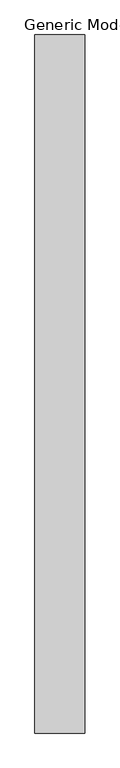
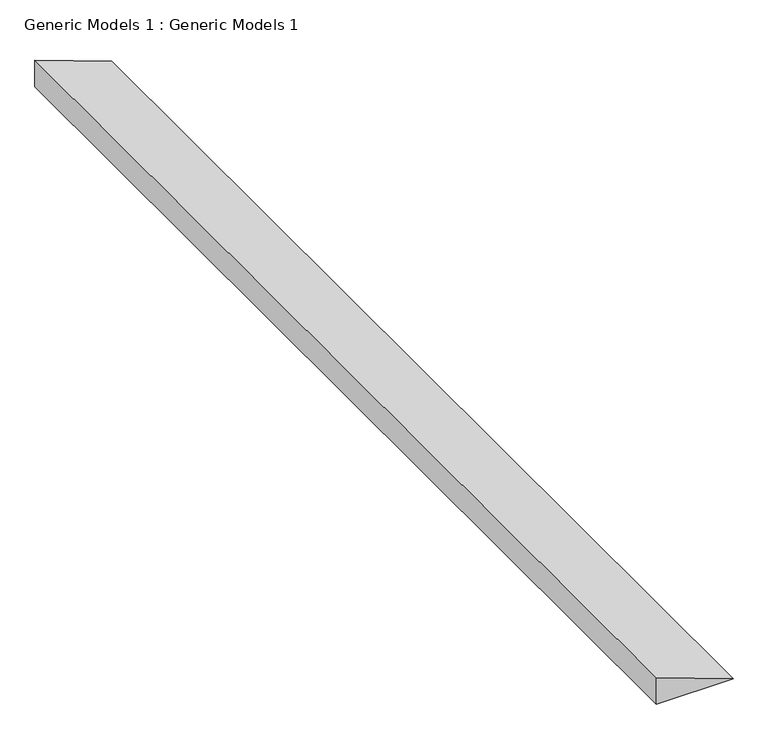
"""IFC4 building model written with IfcOpenShell, lengths in millimetres: proxy geometry, Generic Models 1 : Generic Models 1."""

from ifc_helpers import new_model, si_unit, frame, origin, place, context, project, spatial, polyline, outline, extrude, source, transform, mapped, element, save


def generic_models_1_generic_models_1_ebf34461(model_context):
    return source(origin(), model_context, "Body", "SweptSolid", [
        extrude(outline(polyline([(-609.6, 11475.1785285), (-609.6, 13375.2014317), (81.3174193, 11475.1785285), (-609.6, 11475.1785285)])), frame((0.0, -12819.6698206, 0.0), z_axis=(0.0, 1.0, 0.0), x_axis=(0.0, 0.0, 1.0)), (0.0, 0.0, 1.0), 26642.0634191),
    ])


if __name__ == "__main__":
    model = new_model("IFC4")
    model_context = context("Model", 3, world=origin())
    ifc_project = project(units=[si_unit("LENGTHUNIT", "METRE", prefix="MILLI")], contexts=[model_context])
    site = spatial("IfcSite", under=ifc_project)
    building = spatial("IfcBuilding", under=site)
    placement = place(None, origin())
    generic_models_1_generic_models_1_shape = generic_models_1_generic_models_1_ebf34461(model_context)
    element("IfcBuildingElementProxy", 1, Name="Generic Models 1 : Generic Models 1", ObjectType="Generic Models 1 : Generic Models 1", at=placement, inside=building, context=model_context, shape_type="MappedRepresentation", body=[
        mapped(generic_models_1_generic_models_1_shape, transform((0.0, 0.0, 0.0), x_axis=(1.0, 0.0, 0.0), y_axis=(0.0, 1.0, 0.0), z_axis=(0.0, 0.0, 1.0))),
    ])
    save(model, "model.ifc")
